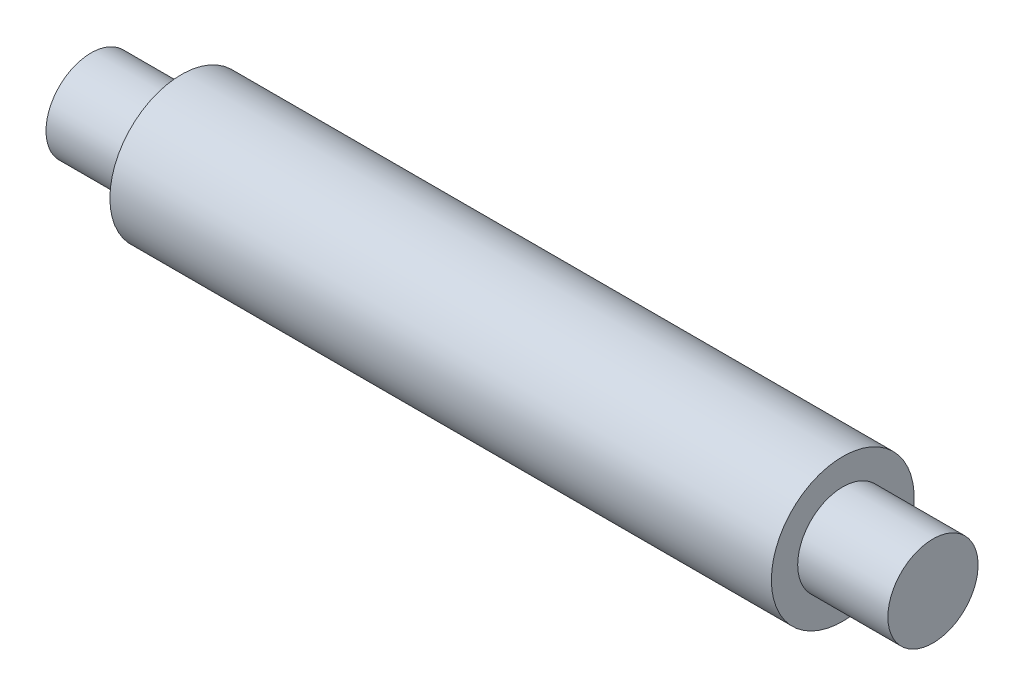
from build123d import *


with BuildPart() as part:
    # Roller Profile Sketch → Roller Body Thin Revolve (revolve)
    with BuildSketch(Plane.XY, mode=Mode.PRIVATE) as roller_body_thin_revolve_sk:
        Polygon((280, 0), (280, 30), (220, 30), (220, 47.5), (-220, 47.5), (-220, 30), (-280, 30), (-280, 0), (-270, 0), (-270, 20), (-210, 20), (-210, 37.5), (210, 37.5), (210, 20), (270, 20), (270, 0), align=None)
    revolve(roller_body_thin_revolve_sk.sketch.rotate(Axis((-409.616293783, 0, 0), (1, 0, 0)), 90), axis=Axis((-409.616293783, 0, 0), (1, 0, 0)))


solid = part.part
